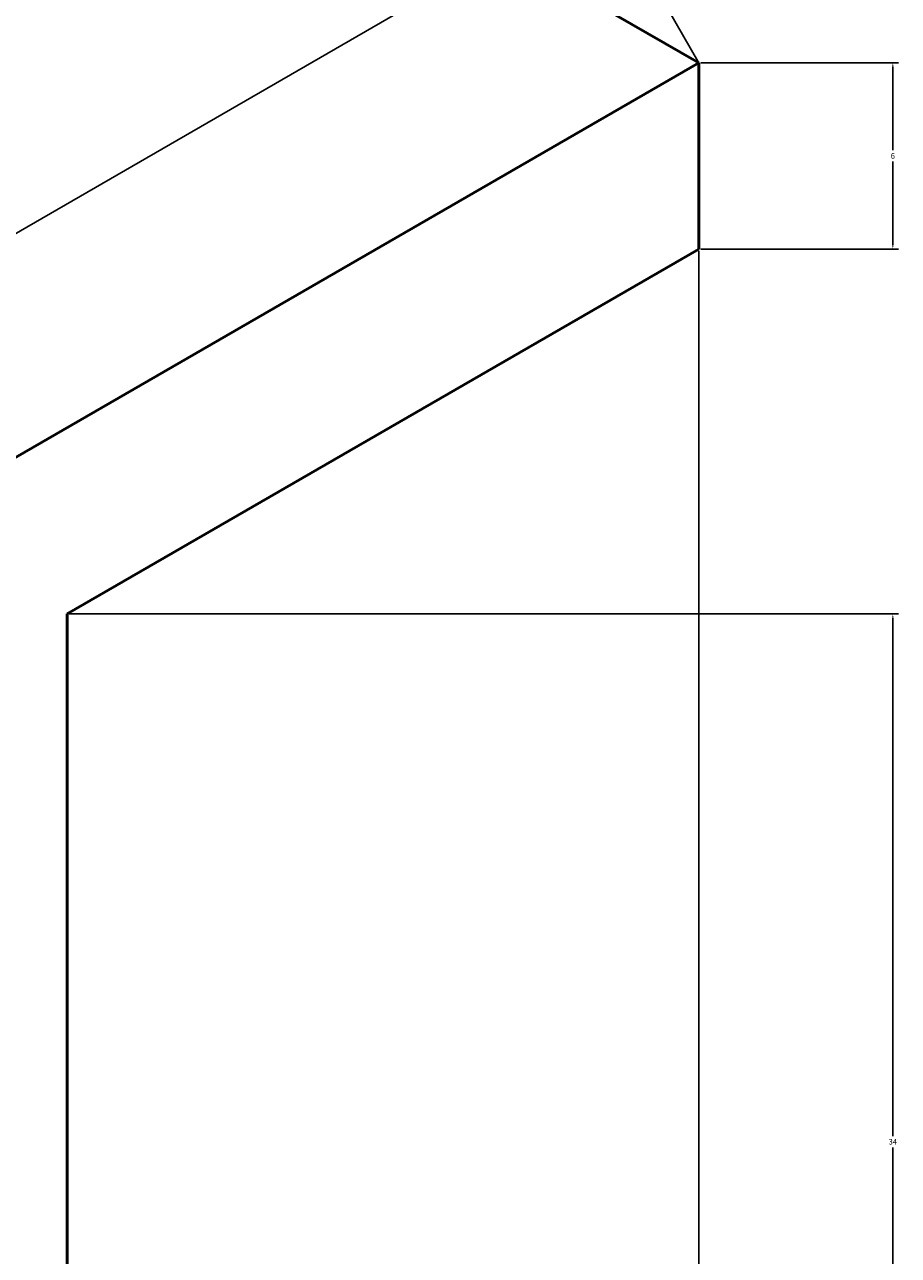
# Model space of a CAD drawing. Units: inches. Extents: x -23 to 69, y -27 to 96.
# Tile 4 of 10: x 40 to 69, y -5 to 35. Entities that reach past the tile are written whole.
import ezdxf

# ---------------------------------------------------------------- set-up
doc = ezdxf.new("R2010")
doc.units = ezdxf.units.IN
doc.header["$MEASUREMENT"] = 0
doc.layers.add('M-DIMS', color=2, linetype='Continuous', lineweight=18)
doc.layers.add('M-OUTL', color=7, linetype='Continuous', lineweight=50)
doc.styles.get("Standard").update_dxf_attribs({"font": 'arial.ttf'})
doc.dimstyles.get("Standard").update_dxf_attribs({"dimtxt": 0.18, "dimasz": 0.18, "dimexe": 0.18, "dimexo": 0.0625, "dimgap": 0.09, "dimtad": 0, "dimtih": 1, "dimtoh": 1, "dimdec": 4, "dimzin": 0, "dimdsep": 46, "dimtxsty": 'Standard', "dimcen": 0.09, "dimadec": 0, "dimazin": 0, "dimtfac": 1, "dimtdec": 4, "dimtofl": 0, "dimtmove": 0, "dimatfit": 3, "dimfxl": 1, "dimtolj": 1, "dimtzin": 0, "dimarcsym": 0})

# ---------------------------------------------------------------- blocks, each defined once
blk = doc.blocks.new('*D1')
at = {"layer": 'Defpoints', "color": 0, "transparency": 16777216}
for p in [(59.046, 39.281), (62.171, 33.869), (16.271, 7.369)]:
    blk.add_point(p, dxfattribs=at)
at = {"layer": 'M-DIMS', "color": 0, "lineweight": -2, "transparency": 16777216}
for p, q in [((62.139, 33.923), (58.956, 39.437)), ((58.89, 39.191), (36.315, 26.158)), ((13.302, 12.871), (35.877, 25.905)), ((16.24, 7.423), (13.056, 12.937))]:
    blk.add_line(p, q, dxfattribs=at)
at = {"layer": 'M-DIMS', "color": 0, "transparency": 16777216}
for points in [[(58.875, 39.217), (58.905, 39.165), (59.046, 39.281)], [(13.287, 12.897), (13.317, 12.845), (13.146, 12.781)]]:
    blk.add_solid(points, dxfattribs=at)
at = {"layer": 'M-DIMS', "color": 0, "transparency": 16777216, "insert": (36.096, 26.031), "char_height": 0.18, "attachment_point": 5}
blk.add_mtext('\\A1;53', dxfattribs=at)
blk = doc.blocks.new('*D3')
at = {"layer": 'Defpoints', "color": 0, "transparency": 16777216}
for p in [(62.171, 33.869), (68.421, 33.869), (62.171, 27.869)]:
    blk.add_point(p, dxfattribs=at)
at = {"layer": 'M-DIMS', "color": 0, "lineweight": -2, "transparency": 16777216}
for p, q in [((62.233, 33.869), (68.601, 33.869)), ((68.421, 33.689), (68.421, 31.051)), ((68.421, 28.049), (68.421, 30.687)), ((62.233, 27.869), (68.601, 27.869))]:
    blk.add_line(p, q, dxfattribs=at)
at = {"layer": 'M-DIMS', "color": 0, "transparency": 16777216}
for points in [[(68.391, 33.689), (68.451, 33.689), (68.421, 33.869)], [(68.391, 28.049), (68.451, 28.049), (68.421, 27.869)]]:
    blk.add_solid(points, dxfattribs=at)
at = {"layer": 'M-DIMS', "color": 0, "transparency": 16777216, "insert": (68.421, 30.869), "char_height": 0.18, "attachment_point": 5}
blk.add_mtext('\\A1;6', dxfattribs=at)
blk = doc.blocks.new('*D4')
at = {"layer": 'Defpoints', "color": 0, "transparency": 16777216}
for p in [(41.819, 16.119), (68.421, 16.119), (41.819, -17.881)]:
    blk.add_point(p, dxfattribs=at)
at = {"layer": 'M-DIMS', "color": 0, "lineweight": -2, "transparency": 16777216}
for p, q in [((41.881, 16.119), (68.601, 16.119)), ((68.421, 15.939), (68.421, -0.699)), ((68.421, -17.701), (68.421, -1.063)), ((41.881, -17.881), (68.601, -17.881))]:
    blk.add_line(p, q, dxfattribs=at)
at = {"layer": 'M-DIMS', "color": 0, "transparency": 16777216}
for points in [[(68.391, 15.939), (68.451, 15.939), (68.421, 16.119)], [(68.391, -17.701), (68.451, -17.701), (68.421, -17.881)]]:
    blk.add_solid(points, dxfattribs=at)
at = {"layer": 'M-DIMS', "color": 0, "transparency": 16777216, "insert": (68.421, -0.881), "char_height": 0.18, "attachment_point": 5}
blk.add_mtext('\\A1;34', dxfattribs=at)
blk = doc.blocks.new('*D17')
at = {"layer": 'Defpoints', "color": 0, "transparency": 16777216}
for p in [(62.171, 27.869), (-16.638, 20.369), (62.171, -27.131)]:
    blk.add_point(p, dxfattribs=at)
at = {"layer": 'M-DIMS', "color": 0, "lineweight": -2, "transparency": 16777216}
for p, q in [((62.171, 27.806), (62.171, -27.311)), ((-16.638, 20.306), (-16.638, -27.311)), ((-16.458, -27.131), (22.391, -27.131)), ((61.991, -27.131), (23.142, -27.131))]:
    blk.add_line(p, q, dxfattribs=at)
at = {"layer": 'M-DIMS', "color": 0, "transparency": 16777216}
for points in [[(-16.458, -27.101), (-16.458, -27.161), (-16.638, -27.131)], [(61.991, -27.101), (61.991, -27.161), (62.171, -27.131)]]:
    blk.add_solid(points, dxfattribs=at)
at = {"layer": 'M-DIMS', "color": 0, "transparency": 16777216, "insert": (22.766, -27.131), "char_height": 0.18, "attachment_point": 5}
blk.add_mtext('\\A1;78.81', dxfattribs=at)

msp = doc.modelspace()

# ---------------------------------------------------------------- linework, layer by layer
at = {"layer": 'M-OUTL'}
for p, q in [((62.1706, 33.8686), (34.4578, 49.8686)), ((16.2712, 7.3686), (62.1706, 33.8686)), ((62.1706, 27.8686), (62.1706, 33.8686)), ((41.819, 16.1186), (62.1706, 27.8686)), ((41.819, -17.8814), (41.819, 16.1186))]:
    msp.add_line(p, q, dxfattribs=at)

# ---------------------------------------------------------------- dimensions: what is measured, and where the dimension line sits
at = {"layer": 'M-DIMS'}
for base, p1, p2, angle, picture, middle in [((59.0456, 39.2813), (16.2712, 7.3686), (62.1706, 33.8686), 30, '*D1', (36.0959, 26.0313)), ((68.4206, 33.8686), (62.1706, 27.8686), (62.1706, 33.8686), 90, '*D3', (68.4206, 30.8686)), ((68.4206, 16.1186), (41.819, -17.8814), (41.819, 16.1186), 90, '*D4', (68.4206, -0.8814))]:
    dim = msp.add_linear_dim(base=base, p1=p1, p2=p2, angle=angle, dimstyle='Standard', override={"dimdec": 0, "dimlfac": 1, "dimrnd": 0, "dimzin": 0, "dimdsep": 46, "dimlunit": 2}, dxfattribs=at)
    dim.commit()
    dim.dimension.update_dxf_attribs({"geometry": picture, "text_midpoint": middle})
dim = msp.add_linear_dim(base=(62.1706, -27.1314), p1=(-16.6377, 20.3686), p2=(62.1706, 27.8686), dimstyle='Standard', override={"dimdec": 2, "dimlfac": 1, "dimrnd": 0, "dimzin": 0, "dimdsep": 46, "dimlunit": 2}, dxfattribs=at)
dim.commit()
dim.dimension.update_dxf_attribs({"geometry": '*D17', "text_midpoint": (22.7664, -27.1314)})

doc.saveas('drawing.dxf')
